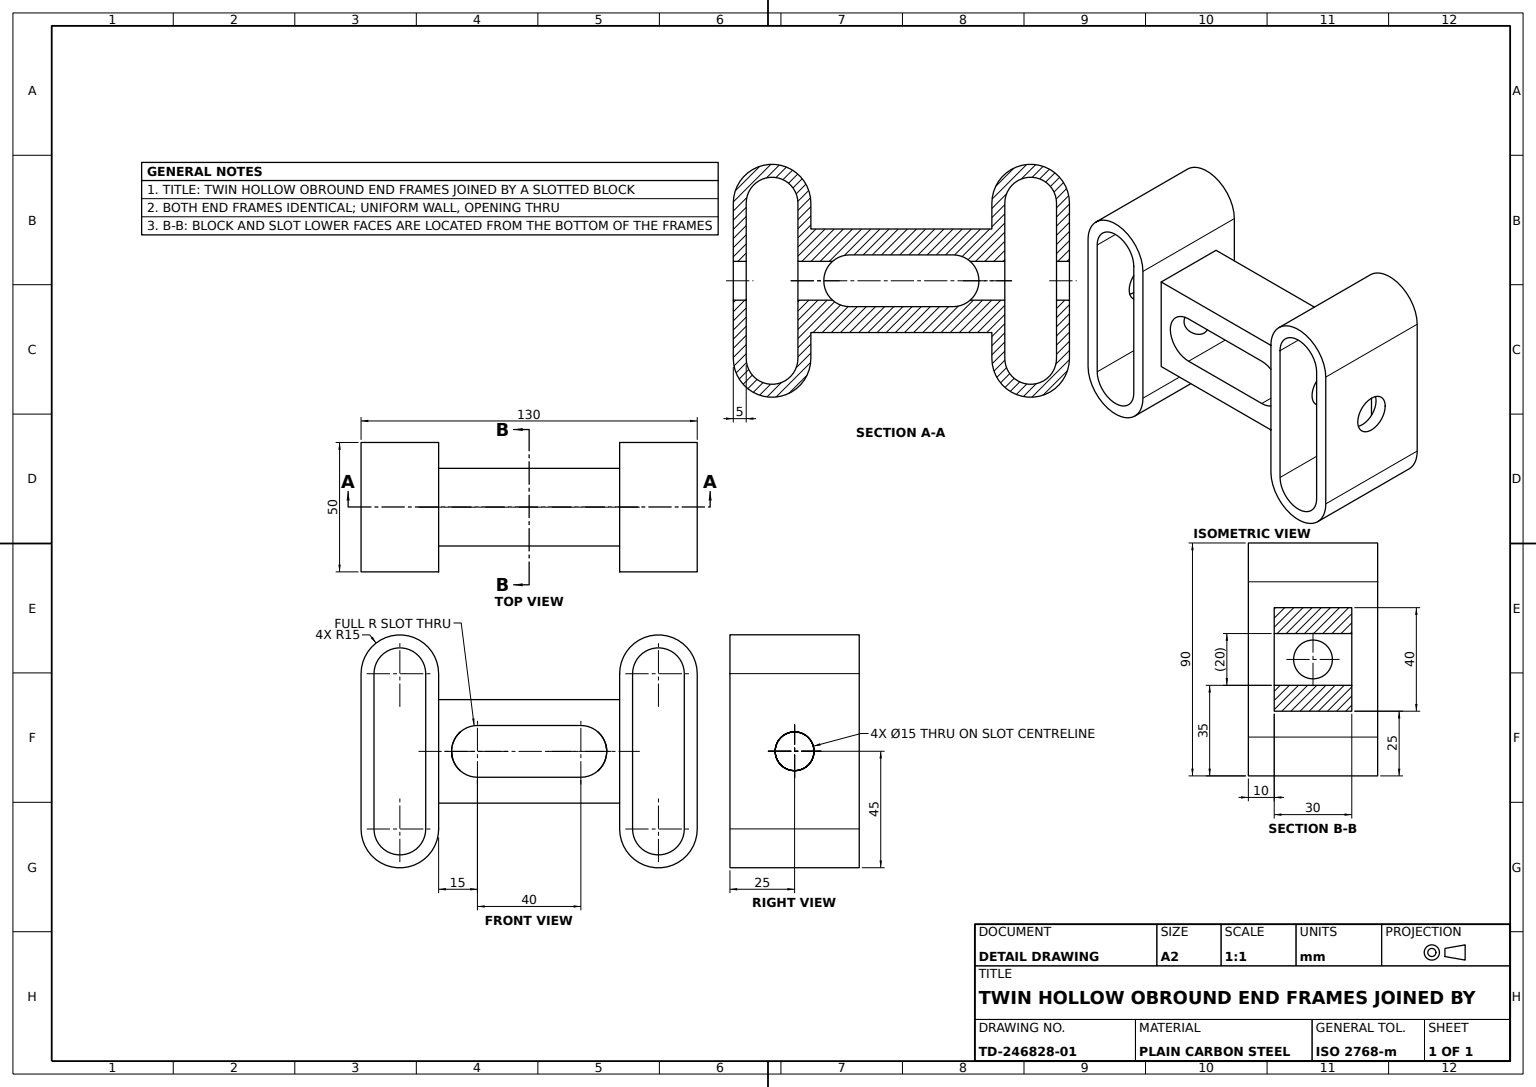
SolidWorks part; units mm, degrees
material "Plain Carbon Steel"
ref_plane "Front Plane" through (0, 0, 0) normal (0, 0, 1) x (1, 0, 0)
ref_plane "Top Plane" through (0, 0, 0) normal (0, 1, 0) x (1, 0, 0)
ref_plane "Right Plane" through (0, 0, 0) normal (1, 0, 0) x (0, 0, -1)
sketch "Centre Block Profile" plane through (0, 0, 0) normal (0, 0, 1) x (1, 0, 0)
  line L0 (-203.1683, 0) -> (198.6139, 0) construction
  line L1 (20, 0) -> (-20, 0) construction
  line L2 (20, -10) -> (-20, -10)
  line L3 (20, 10) -> (-20, 10)
  line L4 (-35, 20) -> (-35, -20)
  line L5 (0, 58.0336) -> (0, -60.4229) construction
  line L6 (35, 20) -> (35, -20)
  line L7 (-35, 20) -> (35, 20)
  line L8 (-35, -20) -> (35, -20)
  arc A0 (20, -10) -> (20, 10) centre (20, 0) ccw
  arc A1 (-20, 10) -> (-20, -10) centre (-20, 0) ccw
  point P5 (0, 0)
  dimension "D1" = 40
  dimension "D2" = 20
  dimension "D3" = 40
  dimension "D4" = 35
extrude "Centre Block" add sketch "Centre Block Profile" along normal blind 30
ref_plane "End Loop Sketch Plane" through (0, 0, 15) normal (0, 0, 1) x (1, 0, 0)
sketch "End Loops Profile" plane through (0, 0, 15) normal (0, 0, 1) x (1, 0, 0)
  line L0 (-77.271, 0) -> (97.1524, 0) construction
  line L1 (50, 30) -> (50, -30) construction
  line L2 (65, 30) -> (65, -30)
  line L3 (35, 30) -> (35, -30)
  line L4 (35, -20) -> (35, 20) construction
  line L5 (60, 30) -> (60, -30)
  line L6 (40, 30) -> (40, -30)
  line L7 (0, 75.0306) -> (0, -56.2226) construction
  line L8 (-50, 30) -> (-50, -30) construction
  line L9 (-65, 30) -> (-65, -30)
  line L10 (-35, 30) -> (-35, -30)
  line L11 (-40, 30) -> (-40, -30)
  line L12 (-60, 30) -> (-60, -30)
  arc A0 (65, 30) -> (35, 30) centre (50, 30) ccw
  arc A1 (35, -30) -> (65, -30) centre (50, -30) ccw
  arc A2 (40, -30) -> (60, -30) centre (50, -30) ccw
  arc A3 (60, 30) -> (40, 30) centre (50, 30) ccw
  arc A4 (-65, 30) -> (-35, 30) centre (-50, 30) cw
  arc A5 (-35, -30) -> (-65, -30) centre (-50, -30) cw
  arc A6 (-60, 30) -> (-40, 30) centre (-50, 30) cw
  arc A7 (-40, -30) -> (-60, -30) centre (-50, -30) cw
  point P6 (50, 0)
  point P11 (50, 45)
  point P12 (50, -45)
  point P25 (-50, 0)
  dimension "D1" = 15
  dimension "D2" = 90
  dimension "D3" = 5
extrude "End Loops" add sketch "End Loops Profile" along normal mid plane 50 contours L3 A1 L2 A0
sketch "Cross Hole Profile" plane through (0, 0, 0) normal (1, 0, 0) x (0, 0, -1)
  line L0 (-15, -45) -> (-15, 47.3438) construction
  line L1 (-40, -45) -> (10, -45) construction
  line L2 (-40, 0) -> (21.4283, 0) construction
  line L3 (-40, -30) -> (-40, 30) construction
  circle A0 centre (-15, 0) radius 7.5
  dimension "D1" = 15
extrude "Cross Hole Ø15" cut sketch "Cross Hole Profile" against normal mid plane 190
